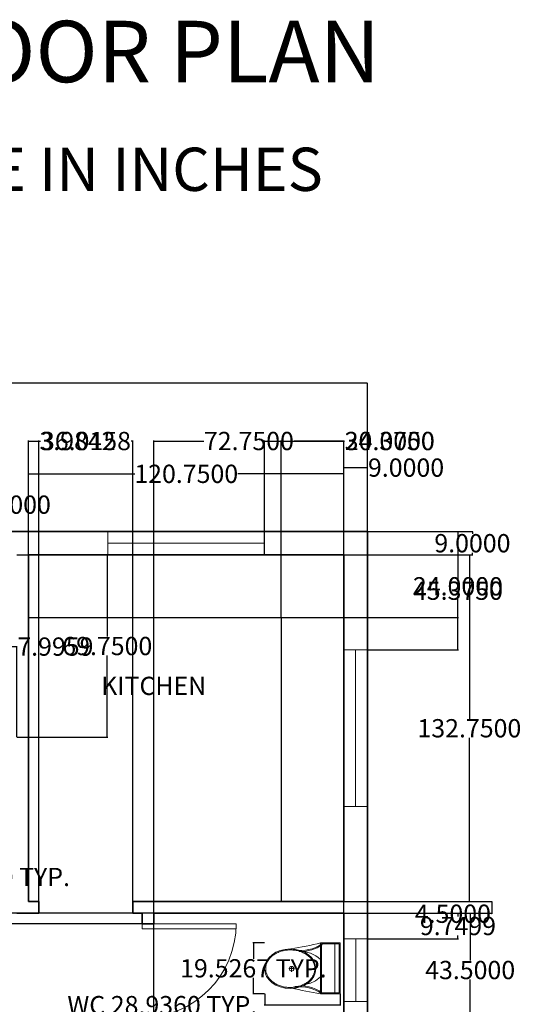
# Model space of a CAD drawing. Units: inches. Extents: x 774 to 2194, y 522 to 1247.
# Tile 6 of 7: x 1088 to 1280, y 870 to 1247. Entities that reach past the tile are written whole.
import ezdxf

# ---------------------------------------------------------------- set-up
doc = ezdxf.new("R2010")
doc.units = ezdxf.units.IN
for name, color, linetype, lineweight in [('A-ANNO-DIMS', 2, 'Continuous', 13), ('A-ANNO-TEXT', 7, 'Continuous', 25), ('A-AREA-IDEN', 3, 'Continuous', 18), ('A-DOOR', 3, 'Continuous', 18), ('A-FLOR-CASE', 9, 'Continuous', 25), ('A-FLOR-FIXT', 7, 'Continuous', 18), ('A-GLAZ', 4, 'Continuous', 18), ('A-WALL', 7, 'Continuous', 35)]:
    doc.layers.add(name, color=color, linetype=linetype, lineweight=lineweight)
doc.styles.get("Standard").update_dxf_attribs({"font": 'arial.ttf'})
doc.dimstyles.get("Standard").update_dxf_attribs({"dimtxt": 7, "dimasz": 0.18, "dimexe": 0.18, "dimexo": 0.0625, "dimgap": 0.09, "dimtad": 0, "dimtih": 1, "dimtoh": 1, "dimdec": 4, "dimzin": 0, "dimdsep": 46, "dimtxsty": 'Standard', "dimcen": 0.09, "dimadec": 0, "dimazin": 0, "dimtfac": 1, "dimtdec": 4, "dimtofl": 0, "dimtmove": 0, "dimatfit": 3, "dimfxl": 1, "dimtolj": 1, "dimtzin": 0, "dimarcsym": 0})

# ---------------------------------------------------------------- blocks, each defined once
blk = doc.blocks.new('A$C31115884')
for p, q in [((258, 466), (258, 523)), ((283, 498), (223, 498)), ((0, 200), (0, 0)), ((520, 200), (0, 200)), ((10, 190), (10, 10)), ((510, 190), (10, 190)), ((510, 10), (510, 190)), ((520, 0), (520, 200)), ((510, 54), (0, 54)), ((10, 10), (510, 10)), ((0, 0), (520, 0))]:
    blk.add_line(p, q)
blk.add_circle((256, 496), 23.6)
for centre, radius, start, end in [((2778, -205), 2807, 165.4549, 171.7133), ((-295, 403), 365, 324.2091, 9.3499), ((-295, 403), 375, 324.2091, 9.3499), ((139, 406), 293, 315.8436, 2.6563), ((806, 403), 375, 179.2036, 215.7909), ((806, 403), 365, 170.6501, 215.7909), ((3237, 905), 2807, 188.2867, 194.5451), ((384, 406), 293, 190.2774, 224.1564)]:
    blk.add_arc(centre, radius, start, end)
blk.add_ellipse((256, 510), major_axis=(0, -261), ratio=0.772727)
blk.add_open_spline([(256, 259), (263, 259), (270, 260), (288, 262), (299, 265), (320, 273), (330, 278), (350, 291), (360, 299), (378, 316), (386, 326), (402, 347), (409, 358), (421, 383), (427, 395), (436, 422), (440, 436), (445, 465), (447, 480), (448, 509), (448, 524), (445, 553), (443, 568), (436, 596), (432, 610), (422, 636), (416, 649), (402, 672), (395, 683), (379, 703), (370, 712), (351, 728), (341, 735), (321, 746), (310, 751), (289, 757), (278, 759), (256, 761), (245, 761), (223, 757), (212, 754), (191, 746), (181, 741), (161, 728), (151, 720), (133, 703), (125, 693), (110, 672), (103, 660), (90, 636), (85, 623), (76, 596), (72, 582), (67, 553), (66, 538), (64, 509), (65, 494), (68, 465), (70, 450), (77, 422), (81, 408), (91, 382), (97, 370), (111, 346), (118, 335), (135, 316), (144, 307), (162, 291), (172, 284), (193, 273), (203, 269), (225, 262), (236, 260), (250, 259), (253, 259), (256, 259)], degree=3, knots=[0, 0, 0, 0, 0.110105, 0.110105, 0.285049, 0.285049, 0.459994, 0.459994, 0.634938, 0.634938, 0.809882, 0.809882, 0.984827, 0.984827, 1.159771, 1.159771, 1.334715, 1.334715, 1.50966, 1.50966, 1.684604, 1.684604, 1.859549, 1.859549, 2.034493, 2.034493, 2.209437, 2.209437, 2.384382, 2.384382, 2.559326, 2.559326, 2.73427, 2.73427, 2.909215, 2.909215, 3.084159, 3.084159, 3.259103, 3.259103, 3.434048, 3.434048, 3.608992, 3.608992, 3.783936, 3.783936, 3.958881, 3.958881, 4.133825, 4.133825, 4.30877, 4.30877, 4.483714, 4.483714, 4.658658, 4.658658, 4.833603, 4.833603, 5.008547, 5.008547, 5.183491, 5.183491, 5.358436, 5.358436, 5.53338, 5.53338, 5.708324, 5.708324, 5.883269, 5.883269, 6.058213, 6.058213, 6.233158, 6.233158, 6.283185, 6.283185, 6.283185, 6.283185])
blk = doc.blocks.new('*D8')
at = {"layer": 'A-ANNO-DIMS', "color": 0, "lineweight": -2, "transparency": 16777216}
for p, q in [((1040.78, 1050.75), (1040.78, 1061.15)), ((1040.96, 1060.97), (1064.6, 1060.97)), ((1064.78, 1050.75), (1064.78, 1061.15)), ((1064.78, 1060.97), (1064.96, 1060.97))]:
    blk.add_line(p, q, dxfattribs=at)
at = {"layer": 'A-ANNO-DIMS', "color": 0, "transparency": 16777216}
for points in [[(1040.96, 1061), (1040.96, 1060.94), (1040.78, 1060.97)], [(1064.6, 1061), (1064.6, 1060.94), (1064.78, 1060.97)]]:
    blk.add_solid(points, dxfattribs=at)
at = {"layer": 'Defpoints', "color": 0, "transparency": 16777216}
for p in [(1064.78, 1060.97), (1040.78, 1050.69), (1064.78, 1050.69)]:
    blk.add_point(p, dxfattribs=at)
at = {"layer": 'A-ANNO-DIMS', "color": 0, "transparency": 16777216, "insert": (1082.35, 1060.97), "char_height": 7, "attachment_point": 5}
blk.add_mtext('\\A1;24.0000', dxfattribs=at)
blk = doc.blocks.new('*D13')
at = {"layer": 'A-ANNO-DIMS', "color": 0, "lineweight": -2, "transparency": 16777216}
for p, q in [((1091.03, 1041.75), (1091.03, 1072.95)), ((1091.21, 1072.77), (1131.69, 1072.77)), ((1211.6, 1072.77), (1171.12, 1072.77)), ((1211.78, 1041.75), (1211.78, 1072.95))]:
    blk.add_line(p, q, dxfattribs=at)
at = {"layer": 'A-ANNO-DIMS', "color": 0, "transparency": 16777216}
for points in [[(1091.21, 1072.8), (1091.21, 1072.74), (1091.03, 1072.77)], [(1211.6, 1072.8), (1211.6, 1072.74), (1211.78, 1072.77)]]:
    blk.add_solid(points, dxfattribs=at)
at = {"layer": 'Defpoints', "color": 0, "transparency": 16777216}
for p in [(1211.78, 1072.77), (1091.03, 1041.69), (1211.78, 1041.69)]:
    blk.add_point(p, dxfattribs=at)
at = {"layer": 'A-ANNO-DIMS', "color": 0, "transparency": 16777216, "insert": (1151.41, 1072.77), "char_height": 7, "attachment_point": 5}
blk.add_mtext('\\A1;120.7500', dxfattribs=at)
blk = doc.blocks.new('*D14')
at = {"layer": 'A-ANNO-DIMS', "color": 0, "lineweight": -2, "transparency": 16777216}
for p, q in [((1211.78, 1041.75), (1211.78, 1075.34)), ((1211.96, 1075.16), (1220.6, 1075.16)), ((1220.78, 1041.75), (1220.78, 1075.34)), ((1220.78, 1075.16), (1220.96, 1075.16))]:
    blk.add_line(p, q, dxfattribs=at)
at = {"layer": 'A-ANNO-DIMS', "color": 0, "transparency": 16777216}
for points in [[(1211.96, 1075.19), (1211.96, 1075.13), (1211.78, 1075.16)], [(1220.6, 1075.19), (1220.6, 1075.13), (1220.78, 1075.16)]]:
    blk.add_solid(points, dxfattribs=at)
at = {"layer": 'Defpoints', "color": 0, "transparency": 16777216}
for p in [(1220.78, 1075.16), (1211.78, 1041.69), (1220.78, 1041.69)]:
    blk.add_point(p, dxfattribs=at)
at = {"layer": 'A-ANNO-DIMS', "color": 0, "transparency": 16777216, "insert": (1235.57, 1075.16), "char_height": 7, "attachment_point": 5}
blk.add_mtext('\\A1;9.0000', dxfattribs=at)
blk = doc.blocks.new('*D15')
at = {"layer": 'A-ANNO-DIMS', "color": 0, "lineweight": -2, "transparency": 16777216}
for p, q in [((860.78, 1053.45), (860.78, 1107.69)), ((860.96, 1107.51), (1020.74, 1107.51)), ((1220.6, 1107.51), (1060.83, 1107.51)), ((1220.78, 1050.75), (1220.78, 1107.69))]:
    blk.add_line(p, q, dxfattribs=at)
at = {"layer": 'A-ANNO-DIMS', "color": 0, "transparency": 16777216}
for points in [[(860.96, 1107.54), (860.96, 1107.48), (860.78, 1107.51)], [(1220.6, 1107.54), (1220.6, 1107.48), (1220.78, 1107.51)]]:
    blk.add_solid(points, dxfattribs=at)
at = {"layer": 'Defpoints', "color": 0, "transparency": 16777216}
for p in [(1220.78, 1107.51), (860.78, 1053.39), (1220.78, 1050.69)]:
    blk.add_point(p, dxfattribs=at)
at = {"layer": 'A-ANNO-DIMS', "color": 0, "transparency": 16777216, "insert": (1040.78, 1107.51), "char_height": 7, "attachment_point": 5}
blk.add_mtext('\\A1;360.0000', dxfattribs=at)
blk = doc.blocks.new('*D23')
at = {"layer": 'A-ANNO-DIMS', "color": 0, "lineweight": -2, "transparency": 16777216}
for p, q in [((1211.84, 1050.69), (1261.16, 1050.69)), ((1260.98, 1050.51), (1260.98, 1049.85)), ((1211.84, 1041.69), (1261.16, 1041.69)), ((1260.98, 1041.87), (1260.98, 1042.52))]:
    blk.add_line(p, q, dxfattribs=at)
at = {"layer": 'A-ANNO-DIMS', "color": 0, "transparency": 16777216}
for points in [[(1260.95, 1050.51), (1261.01, 1050.51), (1260.98, 1050.69)], [(1260.95, 1041.87), (1261.01, 1041.87), (1260.98, 1041.69)]]:
    blk.add_solid(points, dxfattribs=at)
at = {"layer": 'Defpoints', "color": 0, "transparency": 16777216}
for p in [(1211.78, 1050.69), (1211.78, 1041.69), (1260.98, 1041.69)]:
    blk.add_point(p, dxfattribs=at)
at = {"layer": 'A-ANNO-DIMS', "color": 0, "transparency": 16777216, "insert": (1260.98, 1046.19), "char_height": 7, "attachment_point": 5}
blk.add_mtext('\\A1;9.0000', dxfattribs=at)
blk = doc.blocks.new('*D24')
at = {"layer": 'A-ANNO-DIMS', "color": 0, "lineweight": -2, "transparency": 16777216}
for p, q in [((1211.84, 1041.69), (1259.99, 1041.69)), ((1259.81, 1041.51), (1259.81, 978.98)), ((1259.81, 909.12), (1259.81, 971.65)), ((1211.84, 908.94), (1259.99, 908.94))]:
    blk.add_line(p, q, dxfattribs=at)
at = {"layer": 'A-ANNO-DIMS', "color": 0, "transparency": 16777216}
for points in [[(1259.78, 1041.51), (1259.84, 1041.51), (1259.81, 1041.69)], [(1259.78, 909.12), (1259.84, 909.12), (1259.81, 908.94)]]:
    blk.add_solid(points, dxfattribs=at)
at = {"layer": 'Defpoints', "color": 0, "transparency": 16777216}
for p in [(1211.78, 1041.69), (1211.78, 908.94), (1259.81, 908.94)]:
    blk.add_point(p, dxfattribs=at)
at = {"layer": 'A-ANNO-DIMS', "color": 0, "transparency": 16777216, "insert": (1259.81, 975.31), "char_height": 7, "attachment_point": 5}
blk.add_mtext('\\A1;132.7500', dxfattribs=at)
blk = doc.blocks.new('*D25')
at = {"layer": 'A-ANNO-DIMS', "color": 0, "lineweight": -2, "transparency": 16777216}
for p, q in [((1211.84, 908.94), (1268.59, 908.94)), ((1268.41, 908.76), (1268.41, 904.62)), ((1211.84, 904.44), (1268.59, 904.44)), ((1268.41, 904.26), (1268.23, 904.26)), ((1268.41, 904.44), (1268.41, 904.26))]:
    blk.add_line(p, q, dxfattribs=at)
at = {"layer": 'A-ANNO-DIMS', "color": 0, "transparency": 16777216}
for points in [[(1268.38, 908.76), (1268.44, 908.76), (1268.41, 908.94)], [(1268.38, 904.62), (1268.44, 904.62), (1268.41, 904.44)]]:
    blk.add_solid(points, dxfattribs=at)
at = {"layer": 'Defpoints', "color": 0, "transparency": 16777216}
for p in [(1211.78, 908.94), (1211.78, 904.44), (1268.41, 904.44)]:
    blk.add_point(p, dxfattribs=at)
at = {"layer": 'A-ANNO-DIMS', "color": 0, "transparency": 16777216, "insert": (1253.49, 904.26), "char_height": 7, "attachment_point": 5}
blk.add_mtext('\\A1;4.5000', dxfattribs=at)
blk = doc.blocks.new('*D26')
at = {"layer": 'A-ANNO-DIMS', "color": 0, "lineweight": -2, "transparency": 16777216}
for p, q in [((1211.84, 904.44), (1260.29, 904.44)), ((1260.11, 904.26), (1260.11, 886.35)), ((1260.11, 861.12), (1260.11, 879.02)), ((1211.84, 860.94), (1260.29, 860.94))]:
    blk.add_line(p, q, dxfattribs=at)
at = {"layer": 'A-ANNO-DIMS', "color": 0, "transparency": 16777216}
for points in [[(1260.08, 904.26), (1260.14, 904.26), (1260.11, 904.44)], [(1260.08, 861.12), (1260.14, 861.12), (1260.11, 860.94)]]:
    blk.add_solid(points, dxfattribs=at)
at = {"layer": 'Defpoints', "color": 0, "transparency": 16777216}
for p in [(1211.78, 904.44), (1211.78, 860.94), (1260.11, 860.94)]:
    blk.add_point(p, dxfattribs=at)
at = {"layer": 'A-ANNO-DIMS', "color": 0, "transparency": 16777216, "insert": (1260.11, 882.69), "char_height": 7, "attachment_point": 5}
blk.add_mtext('\\A1;43.5000', dxfattribs=at)
blk = doc.blocks.new('DOOR-SWING-36IN')
blk.add_line((36, 0), (36, 2))
blk.add_lwpolyline([(36, 2), (0, 2), (0, 0), (36, 0)], close=True)
blk.add_arc((36, 0), 36, 90, 180)
blk = doc.blocks.new('WIN-60IN-EXT')
for p, q in [((0, 0), (0, 9)), ((60, 0), (60, 9)), ((0, 4.5), (60, 4.5))]:
    blk.add_line(p, q)
blk = doc.blocks.new('WIN-24IN-EXT')
for p, q in [((0, 0), (0, 9)), ((24, 0), (24, 9)), ((0, 4.5), (24, 4.5))]:
    blk.add_line(p, q)
blk = doc.blocks.new('*D40')
at = {"layer": 'A-ANNO-DIMS', "color": 0, "lineweight": -2, "transparency": 16777216}
for p, q in [((982.99, 913), (982.99, 918.52)), ((983.17, 918.34), (1018.81, 918.34)), ((1018.99, 913), (1018.99, 918.52)), ((1018.99, 918.34), (1019.17, 918.34))]:
    blk.add_line(p, q, dxfattribs=at)
at = {"layer": 'A-ANNO-DIMS', "color": 0, "transparency": 16777216}
for points in [[(983.17, 918.37), (983.17, 918.31), (982.99, 918.34)], [(1018.81, 918.37), (1018.81, 918.31), (1018.99, 918.34)]]:
    blk.add_solid(points, dxfattribs=at)
at = {"layer": 'Defpoints', "color": 0, "transparency": 16777216}
for p in [(1018.99, 918.34), (982.99, 912.94), (1018.99, 912.94)]:
    blk.add_point(p, dxfattribs=at)
at = {"layer": 'A-ANNO-DIMS', "color": 0, "transparency": 16777216, "insert": (1064.39, 918.34), "char_height": 7, "attachment_point": 5}
blk.add_mtext('\\A1;DOOR 36.0000 TYP.', dxfattribs=at)
blk = doc.blocks.new('*D44')
at = {"layer": 'A-ANNO-DIMS', "color": 0, "lineweight": -2, "transparency": 16777216}
for p, q in [((1181.45, 873.52), (1181.45, 869.06)), ((1210.39, 873.52), (1210.39, 869.06)), ((1181.45, 869.24), (1181.27, 869.24)), ((1210.21, 869.24), (1181.63, 869.24))]:
    blk.add_line(p, q, dxfattribs=at)
at = {"layer": 'A-ANNO-DIMS', "color": 0, "transparency": 16777216}
for points in [[(1181.63, 869.27), (1181.63, 869.21), (1181.45, 869.24)], [(1210.21, 869.27), (1210.21, 869.21), (1210.39, 869.24)]]:
    blk.add_solid(points, dxfattribs=at)
at = {"layer": 'Defpoints', "color": 0, "transparency": 16777216}
for p in [(1181.45, 873.58), (1210.39, 873.58), (1181.45, 869.24)]:
    blk.add_point(p, dxfattribs=at)
at = {"layer": 'A-ANNO-DIMS', "color": 0, "transparency": 16777216, "insert": (1142.26, 869.24), "char_height": 7, "attachment_point": 5}
blk.add_mtext('\\A1;WC 28.9360 TYP.', dxfattribs=at)
blk = doc.blocks.new('*D45')
at = {"layer": 'A-ANNO-DIMS', "color": 0, "lineweight": -2, "transparency": 16777216}
for p, q in [((1181.39, 893.11), (1176.93, 893.11)), ((1177.11, 892.93), (1177.11, 887.01)), ((1177.11, 873.76), (1177.11, 879.68)), ((1181.39, 873.58), (1176.93, 873.58))]:
    blk.add_line(p, q, dxfattribs=at)
at = {"layer": 'A-ANNO-DIMS', "color": 0, "transparency": 16777216}
for points in [[(1177.08, 892.93), (1177.14, 892.93), (1177.11, 893.11)], [(1177.08, 873.76), (1177.14, 873.76), (1177.11, 873.58)]]:
    blk.add_solid(points, dxfattribs=at)
at = {"layer": 'Defpoints', "color": 0, "transparency": 16777216}
for p in [(1177.11, 893.11), (1181.45, 893.11), (1181.45, 873.58)]:
    blk.add_point(p, dxfattribs=at)
at = {"layer": 'A-ANNO-DIMS', "color": 0, "transparency": 16777216, "insert": (1177.11, 883.35), "char_height": 7, "attachment_point": 5}
blk.add_mtext('\\A1;19.5267 TYP.', dxfattribs=at)
blk = doc.blocks.new('*D50')
at = {"layer": 'A-ANNO-DIMS', "color": 0, "lineweight": -2, "transparency": 16777216}
for p, q in [((1139.03, 861), (1139.03, 1085.52)), ((1139.21, 1085.34), (1158.11, 1085.34)), ((1211.6, 1085.34), (1192.7, 1085.34)), ((1211.78, 861), (1211.78, 1085.52))]:
    blk.add_line(p, q, dxfattribs=at)
at = {"layer": 'A-ANNO-DIMS', "color": 0, "transparency": 16777216}
for points in [[(1139.21, 1085.37), (1139.21, 1085.31), (1139.03, 1085.34)], [(1211.6, 1085.37), (1211.6, 1085.31), (1211.78, 1085.34)]]:
    blk.add_solid(points, dxfattribs=at)
at = {"layer": 'Defpoints', "color": 0, "transparency": 16777216}
for p in [(1211.78, 1085.34), (1139.03, 860.94), (1211.78, 860.94)]:
    blk.add_point(p, dxfattribs=at)
at = {"layer": 'A-ANNO-DIMS', "color": 0, "transparency": 16777216, "insert": (1175.41, 1085.34), "char_height": 7, "attachment_point": 5}
blk.add_mtext('\\A1;72.7500', dxfattribs=at)
blk = doc.blocks.new('*D60')
at = {"layer": 'A-ANNO-DIMS', "color": 0, "lineweight": -2, "transparency": 16777216}
for p, q in [((1181.41, 1041.75), (1181.41, 1085.52)), ((1181.59, 1085.34), (1211.6, 1085.34)), ((1211.78, 1041.75), (1211.78, 1085.52)), ((1211.78, 1085.34), (1211.96, 1085.34))]:
    blk.add_line(p, q, dxfattribs=at)
at = {"layer": 'A-ANNO-DIMS', "color": 0, "transparency": 16777216}
for points in [[(1181.59, 1085.37), (1181.59, 1085.31), (1181.41, 1085.34)], [(1211.6, 1085.37), (1211.6, 1085.31), (1211.78, 1085.34)]]:
    blk.add_solid(points, dxfattribs=at)
at = {"layer": 'Defpoints', "color": 0, "transparency": 16777216}
for p in [(1211.78, 1085.34), (1181.41, 1041.69), (1211.78, 1041.69)]:
    blk.add_point(p, dxfattribs=at)
at = {"layer": 'A-ANNO-DIMS', "color": 0, "transparency": 16777216, "insert": (1229.29, 1085.34), "char_height": 7, "attachment_point": 5}
blk.add_mtext('\\A1;30.3750', dxfattribs=at)
blk = doc.blocks.new('*D63')
at = {"layer": 'A-ANNO-DIMS', "color": 0, "lineweight": -2, "transparency": 16777216}
for p, q in [((1220.84, 1050.69), (1255.61, 1050.69)), ((1255.43, 1050.51), (1255.43, 1031.67)), ((1255.43, 1005.49), (1255.43, 1024.33)), ((1220.84, 1005.31), (1255.61, 1005.31))]:
    blk.add_line(p, q, dxfattribs=at)
at = {"layer": 'A-ANNO-DIMS', "color": 0, "transparency": 16777216}
for points in [[(1255.4, 1050.51), (1255.46, 1050.51), (1255.43, 1050.69)], [(1255.4, 1005.49), (1255.46, 1005.49), (1255.43, 1005.31)]]:
    blk.add_solid(points, dxfattribs=at)
at = {"layer": 'Defpoints', "color": 0, "transparency": 16777216}
for p in [(1220.78, 1050.69), (1255.43, 1050.69), (1220.78, 1005.31)]:
    blk.add_point(p, dxfattribs=at)
at = {"layer": 'A-ANNO-DIMS', "color": 0, "transparency": 16777216, "insert": (1255.43, 1028), "char_height": 7, "attachment_point": 5}
blk.add_mtext('\\A1;45.3750', dxfattribs=at)
blk = doc.blocks.new('*D65')
at = {"layer": 'A-ANNO-DIMS', "color": 0, "lineweight": -2, "transparency": 16777216}
for p, q in [((1211.84, 904.44), (1255.61, 904.44)), ((1255.43, 904.26), (1255.43, 903.23)), ((1220.84, 894.69), (1255.61, 894.69)), ((1255.43, 894.87), (1255.43, 895.9))]:
    blk.add_line(p, q, dxfattribs=at)
at = {"layer": 'A-ANNO-DIMS', "color": 0, "transparency": 16777216}
for points in [[(1255.4, 904.26), (1255.46, 904.26), (1255.43, 904.44)], [(1255.4, 894.87), (1255.46, 894.87), (1255.43, 894.69)]]:
    blk.add_solid(points, dxfattribs=at)
at = {"layer": 'Defpoints', "color": 0, "transparency": 16777216}
for p in [(1211.78, 904.44), (1255.43, 904.44), (1220.78, 894.69)]:
    blk.add_point(p, dxfattribs=at)
at = {"layer": 'A-ANNO-DIMS', "color": 0, "transparency": 16777216, "insert": (1255.43, 899.56), "char_height": 7, "attachment_point": 5}
blk.add_mtext('\\A1;9.7499', dxfattribs=at)
blk = doc.blocks.new('*D67')
at = {"layer": 'A-ANNO-DIMS', "color": 0, "lineweight": -2, "transparency": 16777216}
for p, q in [((1091.09, 1041.69), (1255.61, 1041.69)), ((1255.43, 1041.51), (1255.43, 1033.35)), ((1255.43, 1017.87), (1255.43, 1026.02)), ((1091.09, 1017.69), (1255.61, 1017.69))]:
    blk.add_line(p, q, dxfattribs=at)
at = {"layer": 'A-ANNO-DIMS', "color": 0, "transparency": 16777216}
for points in [[(1255.4, 1041.51), (1255.46, 1041.51), (1255.43, 1041.69)], [(1255.4, 1017.87), (1255.46, 1017.87), (1255.43, 1017.69)]]:
    blk.add_solid(points, dxfattribs=at)
at = {"layer": 'Defpoints', "color": 0, "transparency": 16777216}
for p in [(1091.03, 1041.69), (1091.03, 1017.69), (1255.43, 1017.69)]:
    blk.add_point(p, dxfattribs=at)
at = {"layer": 'A-ANNO-DIMS', "color": 0, "transparency": 16777216, "insert": (1255.43, 1029.69), "char_height": 7, "attachment_point": 5}
blk.add_mtext('\\A1;24.0000', dxfattribs=at)
blk = doc.blocks.new('*D68')
at = {"layer": 'A-ANNO-DIMS', "color": 0, "lineweight": -2, "transparency": 16777216}
for p, q in [((1187.78, 1017.75), (1187.78, 1085.52)), ((1187.96, 1085.34), (1211.6, 1085.34)), ((1211.78, 1041.75), (1211.78, 1085.52)), ((1211.78, 1085.34), (1211.96, 1085.34))]:
    blk.add_line(p, q, dxfattribs=at)
at = {"layer": 'A-ANNO-DIMS', "color": 0, "transparency": 16777216}
for points in [[(1187.96, 1085.37), (1187.96, 1085.31), (1187.78, 1085.34)], [(1211.6, 1085.37), (1211.6, 1085.31), (1211.78, 1085.34)]]:
    blk.add_solid(points, dxfattribs=at)
at = {"layer": 'Defpoints', "color": 0, "transparency": 16777216}
for p in [(1211.78, 1085.34), (1211.78, 1041.69), (1187.78, 1017.69)]:
    blk.add_point(p, dxfattribs=at)
at = {"layer": 'A-ANNO-DIMS', "color": 0, "transparency": 16777216, "insert": (1229.35, 1085.34), "char_height": 7, "attachment_point": 5}
blk.add_mtext('\\A1;24.0000', dxfattribs=at)
blk = doc.blocks.new('*D69')
at = {"layer": 'A-ANNO-DIMS', "color": 0, "lineweight": -2, "transparency": 16777216}
for p, q in [((1095.02, 909), (1095.02, 1085.52)), ((1095.2, 1085.34), (1095.68, 1085.34)), ((1130.85, 1085.34), (1130.37, 1085.34)), ((1131.03, 909), (1131.03, 1085.52))]:
    blk.add_line(p, q, dxfattribs=at)
at = {"layer": 'A-ANNO-DIMS', "color": 0, "transparency": 16777216}
for points in [[(1095.2, 1085.37), (1095.2, 1085.31), (1095.02, 1085.34)], [(1130.85, 1085.37), (1130.85, 1085.31), (1131.03, 1085.34)]]:
    blk.add_solid(points, dxfattribs=at)
at = {"layer": 'Defpoints', "color": 0, "transparency": 16777216}
for p in [(1131.03, 1085.34), (1095.02, 908.94), (1131.03, 908.94)]:
    blk.add_point(p, dxfattribs=at)
at = {"layer": 'A-ANNO-DIMS', "color": 0, "transparency": 16777216, "insert": (1113.02, 1085.34), "char_height": 7, "attachment_point": 5}
blk.add_mtext('\\A1;36.0158', dxfattribs=at)
blk = doc.blocks.new('*D70')
at = {"layer": 'A-ANNO-DIMS', "color": 0, "lineweight": -2, "transparency": 16777216}
for p, q in [((1091.03, 909), (1091.03, 1085.52)), ((1091.21, 1085.34), (1094.84, 1085.34)), ((1095.02, 909), (1095.02, 1085.52)), ((1095.02, 1085.34), (1095.2, 1085.34))]:
    blk.add_line(p, q, dxfattribs=at)
at = {"layer": 'A-ANNO-DIMS', "color": 0, "transparency": 16777216}
for points in [[(1091.21, 1085.37), (1091.21, 1085.31), (1091.03, 1085.34)], [(1094.84, 1085.37), (1094.84, 1085.31), (1095.02, 1085.34)]]:
    blk.add_solid(points, dxfattribs=at)
at = {"layer": 'Defpoints', "color": 0, "transparency": 16777216}
for p in [(1095.02, 1085.34), (1091.03, 908.94), (1095.02, 908.94)]:
    blk.add_point(p, dxfattribs=at)
at = {"layer": 'A-ANNO-DIMS', "color": 0, "transparency": 16777216, "insert": (1109.78, 1085.34), "char_height": 7, "attachment_point": 5}
blk.add_mtext('\\A1;3.9842', dxfattribs=at)
blk = doc.blocks.new('*D72')
at = {"layer": 'A-ANNO-DIMS', "color": 0, "lineweight": -2, "transparency": 16777216}
for p, q in [((1138.97, 904.44), (825.95, 904.44)), ((826.13, 904.44), (826.13, 904.62)), ((826.13, 904.62), (826.31, 904.62)), ((826.13, 900.62), (826.13, 904.26)), ((1138.97, 900.44), (825.95, 900.44))]:
    blk.add_line(p, q, dxfattribs=at)
at = {"layer": 'A-ANNO-DIMS', "color": 0, "transparency": 16777216}
for points in [[(826.1, 904.26), (826.16, 904.26), (826.13, 904.44)], [(826.1, 900.62), (826.16, 900.62), (826.13, 900.44)]]:
    blk.add_solid(points, dxfattribs=at)
at = {"layer": 'Defpoints', "color": 0, "transparency": 16777216}
for p in [(826.13, 904.44), (1139.03, 904.44), (1139.03, 900.44)]:
    blk.add_point(p, dxfattribs=at)
at = {"layer": 'A-ANNO-DIMS', "color": 0, "transparency": 16777216, "insert": (841.06, 904.62), "char_height": 7, "attachment_point": 5}
blk.add_mtext('\\A1;4.0000', dxfattribs=at)
blk = doc.blocks.new('*D75')
at = {"layer": 'A-ANNO-DIMS', "color": 0, "lineweight": -2, "transparency": 16777216}
for p, q in [((1078.54, 972), (1078.54, 1006.77)), ((1078.72, 1006.59), (1086.35, 1006.59)), ((1086.53, 972), (1086.53, 1006.77)), ((1086.53, 1006.59), (1086.71, 1006.59))]:
    blk.add_line(p, q, dxfattribs=at)
at = {"layer": 'A-ANNO-DIMS', "color": 0, "transparency": 16777216}
for points in [[(1078.72, 1006.62), (1078.72, 1006.56), (1078.54, 1006.59)], [(1086.35, 1006.62), (1086.35, 1006.56), (1086.53, 1006.59)]]:
    blk.add_solid(points, dxfattribs=at)
at = {"layer": 'Defpoints', "color": 0, "transparency": 16777216}
for p in [(1086.53, 1006.59), (1078.54, 971.94), (1086.53, 971.94)]:
    blk.add_point(p, dxfattribs=at)
at = {"layer": 'A-ANNO-DIMS', "color": 0, "transparency": 16777216, "insert": (1101.31, 1006.59), "char_height": 7, "attachment_point": 5}
blk.add_mtext('\\A1;7.9959', dxfattribs=at)
blk = doc.blocks.new('*D77')
at = {"layer": 'A-ANNO-DIMS', "color": 0, "lineweight": -2, "transparency": 16777216}
for p, q in [((1086.59, 1041.69), (1121.36, 1041.69)), ((1121.18, 1041.51), (1121.18, 1010.48)), ((1121.18, 972.12), (1121.18, 1003.15)), ((1086.59, 971.94), (1121.36, 971.94))]:
    blk.add_line(p, q, dxfattribs=at)
at = {"layer": 'A-ANNO-DIMS', "color": 0, "transparency": 16777216}
for points in [[(1121.15, 1041.51), (1121.21, 1041.51), (1121.18, 1041.69)], [(1121.15, 972.12), (1121.21, 972.12), (1121.18, 971.94)]]:
    blk.add_solid(points, dxfattribs=at)
at = {"layer": 'Defpoints', "color": 0, "transparency": 16777216}
for p in [(1086.53, 1041.69), (1086.53, 971.94), (1121.18, 971.94)]:
    blk.add_point(p, dxfattribs=at)
at = {"layer": 'A-ANNO-DIMS', "color": 0, "transparency": 16777216, "insert": (1121.18, 1006.81), "char_height": 7, "attachment_point": 5}
blk.add_mtext('\\A1;69.7500', dxfattribs=at)

msp = doc.modelspace()

# ---------------------------------------------------------------- linework, layer by layer
at = {"layer": 'A-FLOR-CASE'}
for p, q in [((1091.03103, 1017.6875), (1187.78103, 1017.6875)), ((1187.78103, 1017.6875), (1187.78103, 908.9375))]:
    msp.add_line(p, q, dxfattribs=at)
at = {"layer": 'A-WALL'}
for p, q in [((1220.78103, 1050.6875), (860.78103, 1050.6875)), ((860.78103, 1050.6875), (1220.78103, 1050.6875)), ((1088.78103, 1050.6875), (1220.78103, 1050.6875)), ((1220.78103, 570.6875), (1220.78103, 1050.6875)), ((1211.78103, 1041.6875), (1091.03103, 1041.6875)), ((1091.03103, 1041.6875), (1091.03103, 908.9375)), ((1091.03103, 1041.6875), (1211.78103, 1041.6875)), ((1091.03103, 1041.6875), (1211.78103, 1041.6875)), ((1211.78103, 1041.6875), (1211.78103, 908.9375)), ((1211.78103, 908.9375), (1211.78103, 1041.6875)), ((1091.03103, 908.9375), (1095.01519, 908.9375)), ((1095.01519, 908.9375), (1095.01519, 904.4375)), ((1131.03103, 908.9375), (1131.03103, 904.4375)), ((1131.03103, 908.9375), (1211.78103, 908.9375)), ((1136.78103, 908.9375), (1211.78103, 908.9375)), ((1220.78103, 906.6875), (1220.78103, 810.6875)), ((1086.53103, 904.4375), (1091.03103, 904.4375)), ((1091.03103, 904.4375), (1095.01519, 904.4375)), ((1131.03103, 904.4375), (1134.53103, 904.4375)), ((1134.53103, 904.4375), (1134.53103, 900.4375)), ((1139.03103, 904.4375), (1211.78103, 904.4375)), ((1139.03103, 904.4375), (1139.03103, 900.4375)), ((1139.03103, 904.4375), (1211.78103, 904.4375)), ((1211.78103, 904.4375), (1211.78103, 860.9375)), ((1211.78103, 812.93733), (1211.78103, 904.4375)), ((1134.53103, 900.4375), (1139.03103, 900.4375))]:
    msp.add_line(p, q, dxfattribs=at)

# ---------------------------------------------------------------- block references
at = {"layer": 'A-DOOR', "rotation": 180}
msp.add_blockref('DOOR-SWING-36IN', (1170.53061, 900.43709), dxfattribs=at)
at = {"layer": 'A-FLOR-FIXT', "xscale": 0.0375513777956547, "yscale": 0.0375513777956547, "zscale": 0.0375513777956547, "rotation": 89.99999999999999}
msp.add_blockref('A$C31115884', (1210.38834, 873.58267), dxfattribs=at)
at = {"layer": 'A-GLAZ'}
for name, p, rotation in [('WIN-60IN-EXT', (1181.40605, 1050.68701), 180), ('WIN-60IN-EXT', (1220.78053, 945.31248), 89.99999999999996), ('WIN-24IN-EXT', (1211.78152, 894.68784), 269.9999999999981)]:
    msp.add_blockref(name, p, dxfattribs=dict(at, rotation=rotation))

# ---------------------------------------------------------------- texts
at = {"layer": 'A-ANNO-TEXT', "attachment_point": 1}
for s, width, gutter_width, insert, char_height in [('2BHK HOUSE FLOOR PLAN  ', 583.4015262, 117.76408, (828.69716, 1246.32206), 23.5528156), ('ALL DIMENSIONS ARE IN INCHES', 531.0058679, 82.8505, (863.26453, 1197.71591), 16.5701005)]:
    msp.add_mtext_dynamic_manual_height_columns(s, width=width, gutter_width=gutter_width, heights=[0], dxfattribs=dict(at, insert=insert, char_height=char_height))
at = {"layer": 'A-AREA-IDEN', "insert": (1118.84587, 995.03779), "char_height": 6.98828, "attachment_point": 1}
msp.add_mtext_dynamic_manual_height_columns('KITCHEN', width=6.294556, gutter_width=34.9414, heights=[0], dxfattribs=at)

# ---------------------------------------------------------------- dimensions: what is measured, and where the dimension line sits
at = {"layer": 'A-ANNO-DIMS'}
for base, p1, p2, override, picture, middle in [((1220.78103, 1107.50884), (860.78103, 1053.38824), (1220.78103, 1050.6875), {"dimclrd": 0, "dimclre": 0, "dimclrt": 0}, '*D15', (1040.78103, 1107.50884)), ((1095.01519, 1085.3375), (1091.03103, 908.9375), (1095.01519, 908.9375), {"dimdec": 4, "dimlfac": 1, "dimrnd": 0, "dimzin": 0, "dimdsep": 46, "dimlunit": 2}, '*D70', (1109.77701, 1085.3375)), ((1131.03103, 1085.3375), (1095.01519, 908.9375), (1131.03103, 908.9375), {"dimdec": 4, "dimlfac": 1, "dimrnd": 0, "dimzin": 0, "dimdsep": 46, "dimlunit": 2}, '*D69', (1113.02311, 1085.3375)), ((1211.78103, 1085.3375), (1139.03103, 860.9375), (1211.78103, 860.9375), {"dimdec": 4, "dimlfac": 1, "dimrnd": 0, "dimzin": 0, "dimdsep": 46, "dimlunit": 2}, '*D50', (1175.40603, 1085.3375)), ((1211.78103, 1085.3375), (1181.40603, 1041.6875), (1211.78103, 1041.6875), {"dimdec": 4, "dimlfac": 1, "dimrnd": 0, "dimzin": 0, "dimdsep": 46, "dimlunit": 2}, '*D60', (1229.28602, 1085.3375)), ((1211.78103, 1085.3375), (1187.78103, 1017.6875), (1211.78103, 1041.6875), {"dimdec": 4, "dimlfac": 1, "dimrnd": 0, "dimzin": 0, "dimdsep": 46, "dimlunit": 2}, '*D68', (1229.34809, 1085.3375)), ((1220.78103, 1075.16038), (1211.78103, 1041.6875), (1220.78103, 1041.6875), {"dimclrd": 0, "dimclre": 0, "dimclrt": 0}, '*D14', (1235.5691, 1075.16038)), ((1211.78103, 1072.76879), (1091.03103, 1041.6875), (1211.78103, 1041.6875), {"dimclrd": 0, "dimclre": 0, "dimclrt": 0}, '*D13', (1151.40603, 1072.76879)), ((1064.78225, 1060.97203), (1040.78225, 1050.6875), (1064.78225, 1050.6875), {"dimclrd": 0, "dimclre": 0, "dimclrt": 0}, '*D8', (1082.34932, 1060.97203)), ((1086.53103, 1006.5875), (1078.53512, 971.9375), (1086.53103, 971.9375), {"dimdec": 4, "dimlfac": 1, "dimrnd": 0, "dimzin": 0, "dimdsep": 46, "dimlunit": 2}, '*D75', (1101.30955, 1006.5875))]:
    dim = msp.add_linear_dim(base=base, p1=p1, p2=p2, dimstyle='Standard', override=override, dxfattribs=at)
    dim.commit()
    dim.dimension.update_dxf_attribs({"geometry": picture, "text_midpoint": middle})
for base, p1, p2, angle, override, picture, middle in [((1260.98161, 1041.6875), (1211.78103, 1050.6875), (1211.78103, 1041.6875), 90, {"dimclrd": 0, "dimclre": 0, "dimclrt": 0}, '*D23', (1260.98161, 1046.1875)), ((1255.43103, 1050.6875), (1220.78103, 1005.3125), (1220.78103, 1050.6875), 90, {"dimdec": 4, "dimlfac": 1, "dimrnd": 0, "dimzin": 0, "dimdsep": 46, "dimlunit": 2}, '*D63', (1255.43103, 1028)), ((1121.18103, 971.9375), (1086.53103, 1041.6875), (1086.53103, 971.9375), 270, {"dimdec": 4, "dimlfac": 1, "dimrnd": 0, "dimzin": 0, "dimdsep": 46, "dimlunit": 2}, '*D77', (1121.18103, 1006.8125)), ((1255.43103, 1017.6875), (1091.03103, 1041.6875), (1091.03103, 1017.6875), 90, {"dimdec": 4, "dimlfac": 1, "dimrnd": 0, "dimzin": 0, "dimdsep": 46, "dimlunit": 2}, '*D67', (1255.43103, 1029.6875)), ((1259.81484, 908.9375), (1211.78103, 1041.6875), (1211.78103, 908.9375), 90, {"dimclrd": 0, "dimclre": 0, "dimclrt": 0}, '*D24', (1259.81484, 975.3125)), ((826.13103, 904.4375), (1139.03103, 900.4375), (1139.03103, 904.4375), 90, {"dimdec": 4, "dimlfac": 1, "dimrnd": 0, "dimzin": 0, "dimdsep": 46, "dimlunit": 2}, '*D72', (841.05996, 904.6175)), ((1268.41456, 904.4375), (1211.78103, 908.9375), (1211.78103, 904.4375), 90, {"dimclrd": 0, "dimclre": 0, "dimclrt": 0}, '*D25', (1253.48562, 904.2575)), ((1260.11063, 860.9375), (1211.78103, 904.4375), (1211.78103, 860.9375), 90, {"dimclrd": 0, "dimclre": 0, "dimclrt": 0}, '*D26', (1260.11063, 882.6875)), ((1255.43103, 904.4375), (1220.78103, 894.68759), (1211.78103, 904.4375), 90, {"dimdec": 4, "dimlfac": 1, "dimrnd": 0, "dimzin": 0, "dimdsep": 46, "dimlunit": 2}, '*D65', (1255.43103, 899.56254))]:
    dim = msp.add_linear_dim(base=base, p1=p1, p2=p2, angle=angle, dimstyle='Standard', override=override, dxfattribs=at)
    dim.commit()
    dim.dimension.update_dxf_attribs({"geometry": picture, "text_midpoint": middle})
dim = msp.add_linear_dim(base=(1018.99358, 918.33658), p1=(982.99358, 912.93658), p2=(1018.99358, 912.93658), text='DOOR <> TYP.', dimstyle='Standard', override={"dimdec": 4, "dimlfac": 1, "dimrnd": 0, "dimzin": 0, "dimdsep": 46, "dimlunit": 2}, dxfattribs=at)
dim.commit()
dim.dimension.update_dxf_attribs({"geometry": '*D40', "text_midpoint": (1064.38875, 918.33658)})
for base, p1, p2, angle, text, picture, middle in [((1177.11198, 893.10939), (1181.45237, 873.58267), (1181.45237, 893.10939), 90, '<> TYP.', '*D45', (1177.11198, 883.34603)), ((1181.45237, 869.24227), (1210.38834, 873.58267), (1181.45237, 873.58267), 180, 'WC <> TYP.', '*D44', (1142.26218, 869.24227))]:
    dim = msp.add_linear_dim(base=base, p1=p1, p2=p2, angle=angle, text=text, dimstyle='Standard', override={"dimdec": 4, "dimlfac": 1, "dimrnd": 0, "dimzin": 0, "dimdsep": 46, "dimlunit": 2}, dxfattribs=at)
    dim.commit()
    dim.dimension.update_dxf_attribs({"geometry": picture, "text_midpoint": middle})

doc.saveas('drawing.dxf')
